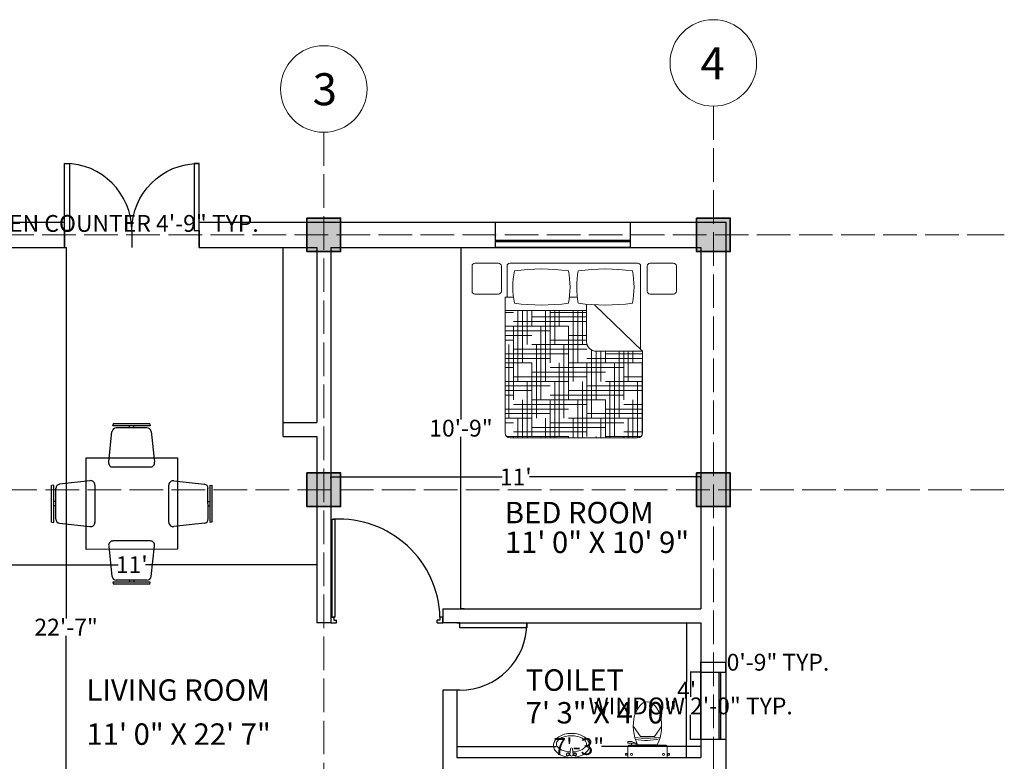
# Model space of a CAD drawing. Units: inches. Extents: x -113 to 5399, y -1393 to 3302.
# Tile 40 of 40: x 3412 to 3763, y 3038 to 3302. Entities that reach past the tile are written whole.
import ezdxf

# ---------------------------------------------------------------- set-up
doc = ezdxf.new("R2010")
doc.units = ezdxf.units.IN
doc.header["$MEASUREMENT"] = 0
doc.linetypes.add('ACAD_ISO02W100', pattern=[15, 12, -3])
for name, color, linetype, lineweight in [('A-ANNO-DIMS', 254, 'Continuous', 18), ('A-AREA-IDEN', 4, 'Continuous', 18), ('A-COLS', 7, 'Continuous', 35), ('A-FLOR-FIXT', 8, 'Continuous', 18), ('A-GRID-IDEN', 7, 'Continuous', 18), ('doors', 2, 'Continuous', 25), ('furniture', 131, 'Continuous', 18), ('GRIDS', 7, 'ACAD_ISO02W100', 13), ('walls', 1, 'Continuous', 25), ('windows', 3, 'Continuous', 25)]:
    doc.layers.add(name, color=color, linetype=linetype, lineweight=lineweight)
doc.layers.add('B-FURNITURE', color=22, linetype='Continuous')
doc.styles.get("Standard").update_dxf_attribs({"font": 'arial.ttf'})
doc.dimstyles.get("Standard").update_dxf_attribs({"dimtxt": 6, "dimasz": 0.18, "dimexe": 0.18, "dimexo": 0.0625, "dimgap": 0.09, "dimtad": 0, "dimtih": 1, "dimtoh": 1, "dimdec": 1, "dimzin": 0, "dimdsep": 46, "dimlunit": 4, "dimtxsty": 'Standard', "dimblk": 'ARCHTICK', "dimcen": 0.09, "dimadec": 0, "dimazin": 0, "dimtfac": 1, "dimtdec": 1, "dimtofl": 0, "dimtmove": 0, "dimatfit": 3, "dimfxl": 1, "dimtolj": 1, "dimtzin": 0, "dimarcsym": 0})

# ---------------------------------------------------------------- blocks, each defined once
blk = doc.blocks.new('*U2')
for p, q in [((0, 0), (0, -6)), ((24, 0), (24, -6))]:
    blk.add_line(p, q)
blk.add_lwpolyline([(0, 0), (0, 24), (1.75, 24), (1.75, 0)], close=True)
blk.add_arc((0, 0), 24, 0, 90)
blk = doc.blocks.new('*X4')
at = {"color": 0}
for p, q in [((4.359, 18.562), (4.359, 18.646)), ((4.453, 17.817), (4.453, 18.562)), ((4.5, 18), (4.5, 18.646)), ((4.5, 18.562), (5.25, 18.562)), ((4.547, 18.188), (4.547, 18.646)), ((4.594, 18.375), (4.594, 18.646)), ((4.641, 18.562), (4.641, 18.646)), ((4.687, 18.609), (5.437, 18.609)), ((4.734, 17.812), (4.734, 18.562)), ((4.781, 18), (4.781, 18.646)), ((4.828, 18.188), (4.828, 18.646)), ((4.875, 18.375), (4.875, 18.646)), ((4.922, 18.562), (4.922, 18.646)), ((5.016, 17.812), (5.016, 18.562)), ((5.062, 18), (5.062, 18.646)), ((5.109, 18.188), (5.109, 18.646)), ((5.156, 18.375), (5.156, 18.646)), ((5.203, 18.562), (5.203, 18.646)), ((5.297, 17.812), (5.297, 18.562)), ((5.344, 18), (5.344, 18.646)), ((5.391, 18.188), (5.391, 18.646)), ((5.437, 18.375), (5.437, 18.646)), ((5.484, 18.562), (5.484, 18.646)), ((5.578, 17.812), (5.578, 18.562)), ((5.625, 18), (5.625, 18.629)), ((5.625, 18.562), (5.637, 18.562)), ((4.34, 18.516), (5.062, 18.516)), ((4.34, 18.469), (4.875, 18.469)), ((5.25, 18.469), (5.637, 18.469)), ((5.437, 18.516), (5.637, 18.516)), ((4.34, 18.422), (4.687, 18.422)), ((4.34, 18.375), (4.5, 18.375)), ((4.406, 17.817), (4.406, 18.375)), ((4.687, 17.811), (4.687, 18.375)), ((4.875, 18.375), (5.625, 18.375)), ((4.969, 17.625), (4.969, 18.375)), ((5.062, 18.422), (5.637, 18.422)), ((5.25, 17.625), (5.25, 18.375)), ((5.531, 17.625), (5.531, 18.375)), ((4.5, 18.281), (5.25, 18.281)), ((4.687, 18.328), (5.437, 18.328)), ((5.625, 18.281), (5.637, 18.281)), ((4.34, 18.234), (5.062, 18.234)), ((4.34, 18.188), (4.875, 18.188)), ((4.359, 17.817), (4.359, 18.188)), ((4.641, 17.817), (4.641, 18.188)), ((4.922, 17.438), (4.922, 18.188)), ((5.203, 17.438), (5.203, 18.188)), ((5.25, 18.188), (5.637, 18.188)), ((5.437, 18.234), (5.637, 18.234)), ((5.484, 17.438), (5.484, 18.188)), ((4.34, 18.141), (4.687, 18.141)), ((4.34, 18.094), (4.5, 18.094)), ((4.875, 18.094), (5.625, 18.094)), ((5.062, 18.141), (5.637, 18.141)), ((4.5, 18), (5.25, 18)), ((4.594, 17.817), (4.594, 18)), ((4.687, 18.047), (5.437, 18.047)), ((4.875, 17.25), (4.875, 18)), ((5.156, 17.25), (5.156, 18)), ((5.437, 17.25), (5.437, 18)), ((5.625, 18), (5.637, 18)), ((4.34, 17.953), (5.062, 17.953)), ((4.34, 17.906), (4.875, 17.906)), ((4.34, 17.859), (4.687, 17.859)), ((5.062, 17.859), (5.637, 17.859)), ((5.25, 17.906), (5.637, 17.906)), ((5.437, 17.953), (5.637, 17.953)), ((4.742, 17.766), (5.437, 17.766)), ((4.828, 17.246), (4.828, 17.812)), ((4.875, 17.812), (5.625, 17.812)), ((5.109, 17.246), (5.109, 17.812)), ((5.391, 17.246), (5.391, 17.812)), ((4.755, 17.719), (5.25, 17.719)), ((4.755, 17.672), (5.062, 17.672)), ((5.437, 17.672), (5.637, 17.672)), ((5.625, 17.719), (5.637, 17.719)), ((4.755, 17.625), (4.875, 17.625)), ((4.781, 17.246), (4.781, 17.625)), ((5.062, 17.246), (5.062, 17.625)), ((5.062, 17.578), (5.637, 17.578)), ((5.25, 17.625), (5.637, 17.625)), ((5.344, 17.246), (5.344, 17.625)), ((5.625, 17.263), (5.625, 17.625)), ((4.755, 17.484), (5.437, 17.484)), ((4.875, 17.531), (5.625, 17.531)), ((4.755, 17.438), (5.25, 17.438)), ((4.755, 17.391), (5.062, 17.391)), ((5.016, 17.246), (5.016, 17.438)), ((5.297, 17.246), (5.297, 17.438)), ((5.437, 17.391), (5.637, 17.391)), ((5.578, 17.246), (5.578, 17.438)), ((5.625, 17.438), (5.637, 17.438)), ((4.755, 17.344), (4.875, 17.344)), ((5.062, 17.297), (5.637, 17.297)), ((5.25, 17.344), (5.637, 17.344)), ((4.875, 17.25), (5.608, 17.25)), ((4.969, 17.246), (4.969, 17.25)), ((5.25, 17.246), (5.25, 17.25)), ((5.531, 17.246), (5.531, 17.25))]:
    blk.add_line(p, q, dxfattribs=at)
blk = doc.blocks.new('MAT-P01')
for p, q in [((-0.021, 0.816), (-0.021, 0.56)), ((0.009, 0.846), (0.247, 0.846)), ((0.277, 0.816), (0.277, 0.56)), ((0.344, 0.816), (0.344, -0.032)), ((0.374, 0.846), (1.674, 0.846)), ((1.704, 0.816), (1.704, 0.5)), ((1.762, 0.816), (1.762, 0.56)), ((1.792, 0.846), (2.031, 0.846)), ((2.061, 0.816), (2.061, 0.56)), ((0.009, 0.53), (0.247, 0.53)), ((1.792, 0.53), (2.031, 0.53)), ((0.815, 0.423), (0.324, -0.051)), ((0.895, 0.429), (0.895, 0.049)), ((0.988, 0.5), (1.069, 0.5)), ((1.639, 0.5), (1.724, 0.5)), ((1.724, 0.5), (1.724, -0.884)), ((0.895, 0.364), (1.724, 0.364)), ((0.895, 0.364), (0.895, 0.049)), ((0.895, 0.364), (1.724, 0.364)), ((1.724, 0.364), (1.724, -0.884)), ((0.324, -0.051), (0.795, -0.051)), ((0.324, -0.051), (0.324, -0.884)), ((0.374, -0.934), (1.674, -0.934))]:
    blk.add_line(p, q)
for centre, radius, start, end in [((0.009, 0.816), 0.03, 90, 180), ((0.247, 0.816), 0.03, 0, 90), ((0.374, 0.816), 0.03, 90, 180), ((1.674, 0.816), 0.03, 0, 90), ((1.792, 0.816), 0.03, 90, 180), ((2.031, 0.816), 0.03, 0, 90), ((1.225, 0.603), 0.814, 168.373, 191.627), ((0.703, -1.144), 1.931, 81.8162, 98.1838), ((0.181, 0.603), 0.814, 348.373, 11.627), ((1.877, 0.603), 0.814, 168.373, 191.627), ((1.354, -1.144), 1.931, 81.8162, 98.1838), ((0.832, 0.603), 0.814, 348.373, 11.627), ((0.009, 0.56), 0.03, 180, 270), ((0.247, 0.56), 0.03, 270, 0), ((1.792, 0.56), 0.03, 180, 270), ((2.031, 0.56), 0.03, 270, 0), ((0.703, 2.35), 1.931, 261.8162, 278.1838), ((1.354, 2.35), 1.931, 261.8162, 278.1838), ((0.795, 0.049), 0.1, 270, 0), ((0.374, -0.884), 0.05, 180, 270), ((1.674, -0.884), 0.05, 270, 0)]:
    blk.add_arc(centre, radius, start, end)
at = {"rotation": 270}
blk.add_blockref('*X4', (-16.922, 4.704), dxfattribs=at)
blk = doc.blocks.new('A$C6ACA79D1')
at = {"layer": 'B-FURNITURE'}
for p, q in [((-0.503, 0.053), (-0.801, -0.244)), ((-0.483, 0.039), (-0.787, -0.264)), ((-0.503, 0.053), (-0.483, 0.039)), ((-0.429, 0), (-0.155, -0.22)), ((0.787, -0.259), (0.483, 0.044)), ((0.484, 0.043), (0.504, 0.058)), ((0.743, -0.249), (0.493, 0)), ((0.801, -0.239), (0.503, 0.059)), ((-0.493, -0.005), (-0.743, -0.254)), ((-0.601, -0.112), (-0.618, -0.095)), ((0.601, -0.107), (0.618, -0.09)), ((-0.635, -0.147), (-0.652, -0.13)), ((0.635, -0.142), (0.652, -0.124)), ((-0.786, -0.264), (-0.8, -0.244)), ((-0.148, -0.296), (-0.451, -0.599)), ((0.451, -0.594), (0.148, -0.291)), ((0.748, -0.313), (0.527, -0.588)), ((0.801, -0.239), (0.787, -0.259)), ((-0.148, -1.194), (-0.451, -0.891)), ((0.451, -0.896), (0.148, -1.199)), ((0.748, -1.177), (0.527, -0.902)), ((-0.786, -1.227), (-0.8, -1.247)), ((-0.483, -1.529), (-0.787, -1.226)), ((-0.493, -1.485), (-0.743, -1.236)), ((0.787, -1.231), (0.483, -1.535)), ((0.743, -1.241), (0.493, -1.49)), ((0.801, -1.251), (0.787, -1.231)), ((-0.503, -1.544), (-0.801, -1.246)), ((-0.635, -1.343), (-0.652, -1.361)), ((-0.429, -1.49), (-0.155, -1.27)), ((0.801, -1.251), (0.503, -1.549)), ((0.635, -1.349), (0.652, -1.366)), ((-0.601, -1.378), (-0.618, -1.395)), ((0.601, -1.383), (0.618, -1.4)), ((-0.503, -1.544), (-0.483, -1.529)), ((0.484, -1.534), (0.504, -1.548))]:
    blk.add_line(p, q, dxfattribs=at)
at = {"layer": 'B-FURNITURE', "ltscale": 300}
for p, q in [((0.155, -0.215), (0.429, 0.005)), ((-0.527, -0.593), (-0.748, -0.319)), ((-0.527, -0.897), (-0.748, -1.172)), ((0.155, -1.275), (0.429, -1.496))]:
    blk.add_line(p, q, dxfattribs=at)
blk.add_lwpolyline([(-0.742, -0.742), (0, 0), (0.742, -0.742), (0, -1.485)], close=True, dxfattribs=at)
at = {"layer": 'B-FURNITURE', "ltscale": 400}
for centre, start, end in [((-0.458, -0.04), 54.4069, 135), ((0.459, -0.036), 45, 125.5931), ((-0.706, -0.289), 135, 215.5931), ((0.707, -0.284), 324.4069, 45), ((-0.706, -1.201), 144.4069, 225), ((0.707, -1.206), 315, 35.5931), ((-0.458, -1.45), 225, 305.5931), ((0.459, -1.454), 234.4069, 315)]:
    blk.add_arc(centre, 0.0499, start, end, dxfattribs=at)
at = {"layer": 'B-FURNITURE', "ltscale": 300}
for centre, start, end in [((-0.184, -0.261), 315, 54.4069), ((0.184, -0.256), 125.5931, 225), ((-0.487, -0.564), 215.5931, 315), ((0.487, -0.559), 225, 324.4069), ((-0.487, -0.926), 45, 144.4069), ((0.487, -0.931), 35.5931, 135), ((-0.184, -1.229), 305.5931, 45), ((0.184, -1.234), 135, 234.4069)]:
    blk.add_arc(centre, 0.05, start, end, dxfattribs=at)
blk = doc.blocks.new('toilet-3')
at = {"color": 0, "linetype": 'ByBlock'}
for p, q in [((-0.281, -0.05), (-0.281, -0.069)), ((-0.281, -0.05), (-0.261, -0.05)), ((-0.281, -0.069), (-0.261, -0.069)), ((-0.261, -0.047), (-0.261, -0.072)), ((-0.261, -0.047), (-0.251, -0.047)), ((-0.261, -0.072), (-0.251, -0.072)), ((-0.251, -0.047), (-0.251, -0.072)), ((-0.25, -0.03), (-0.25, -0.165)), ((0.24, -0.02), (-0.24, -0.02)), ((0.25, -0.03), (0.25, -0.165)), ((0.261, -0.047), (0.251, -0.047)), ((0.251, -0.047), (0.251, -0.072)), ((0.261, -0.072), (0.251, -0.072)), ((0.261, -0.047), (0.261, -0.072)), ((0.281, -0.05), (0.261, -0.05)), ((0.281, -0.069), (0.261, -0.069)), ((0.281, -0.05), (0.281, -0.069)), ((-0.144, -0.2), (-0.25, -0.2)), ((-0.25, -0.2), (-0.25, -0.222)), ((-0.198, -0.222), (-0.25, -0.222)), ((0.24, -0.175), (-0.24, -0.175)), ((-0.202, -0.2), (-0.202, -0.175)), ((-0.198, -0.222), (-0.16, -0.207)), ((-0.16, -0.207), (-0.16, -0.2)), ((-0.144, -0.2), (-0.144, -0.175)), ((0.125, -0.182), (-0.125, -0.182)), ((-0.089, -0.287), (-0.18, -0.415)), ((0.089, -0.287), (-0.089, -0.287)), ((0.089, -0.287), (0.18, -0.415))]:
    blk.add_line(p, q, dxfattribs=at)
for centre in [(-0.205, -0.059), (0.205, -0.059)]:
    blk.add_circle(centre, 0.0125, dxfattribs=at)
for centre, radius, start, end in [((-0.24, -0.03), 0.01, 90, 180), ((0.24, -0.03), 0.01, 0, 90), ((-0.24, -0.165), 0.01, 180, 270), ((0.376, -0.424), 0.557, 154.2321, 193.6755), ((-0.005, -0.896), 0.659, 75.9276, 103.0204), ((-0.376, -0.424), 0.557, 346.3245, 25.7679), ((0.24, -0.165), 0.01, 270, 0), ((-0.013, -1.787), 1.521, 83.4552, 95.5271), ((0.262, -0.406), 0.452, 199.2942, 217.2549), ((-0.265, -0.4), 0.457, 322.2382, 340.1051), ((-0.001, -0.609), 0.12, 216.3794, 323.6206)]:
    blk.add_arc(centre, radius, start, end, dxfattribs=at)
blk = doc.blocks.new('wash-6')
at = {"color": 0, "linetype": 'ByBlock'}
for p, q in [((-0.036, -0.063), (-0.021, -0.18)), ((0.036, -0.063), (0.021, -0.18))]:
    blk.add_line(p, q, dxfattribs=at)
for centre, radius in [((-0.075, -0.062), 0.0325), ((-0.075, -0.062), 0.0263), ((0.075, -0.062), 0.0325), ((0.075, -0.062), 0.0263)]:
    blk.add_circle(centre, radius, dxfattribs=at)
for centre, radius, start, end in [((0, -0.56), 0.56, 90, 105.4371), ((-0.204, -0.25), 0.17, 148.1465, 180), ((-0.107, -0.311), 0.285, 123.6901, 148.1465), ((-0.114, -0.361), 0.225, 118.369, 142.5096), ((-0.042, -0.407), 0.401, 105.4371, 123.6901), ((-0.045, -0.488), 0.37, 102.6081, 118.369), ((0, -0.69), 0.576, 92.9466, 102.6081), ((0, -0.063), 0.0361, 0, 180), ((0, -0.18), 0.0215, 180, 0), ((0, -0.56), 0.56, 74.5629, 90), ((0, -0.69), 0.576, 77.3919, 87.0534), ((0.045, -0.488), 0.37, 61.631, 77.3919), ((0.042, -0.407), 0.401, 56.3099, 74.5629), ((0.114, -0.361), 0.225, 37.4904, 61.631), ((0.107, -0.311), 0.285, 31.8535, 56.3099), ((0.204, -0.25), 0.17, 0, 31.8535), ((-0.204, -0.25), 0.17, 180, 211.8535), ((-0.107, -0.189), 0.285, 211.8535, 236.3099), ((-0.217, -0.282), 0.0954, 142.5096, 180), ((-0.217, -0.282), 0.0954, 180, 217.4904), ((-0.114, -0.203), 0.225, 217.4904, 241.631), ((-0.045, -0.076), 0.37, 241.631, 257.3919), ((0.045, -0.076), 0.37, 282.6081, 298.369), ((0.114, -0.203), 0.225, 298.369, 322.5096), ((0.107, -0.189), 0.285, 303.6901, 328.1465), ((0.217, -0.282), 0.0954, 0, 37.4904), ((0.217, -0.282), 0.0954, 322.5096, 0), ((0.204, -0.25), 0.17, 328.1465, 0), ((-0.042, -0.092), 0.401, 236.3099, 254.5629), ((0, 0.06), 0.56, 254.5629, 270), ((0, 0.125), 0.576, 257.3919, 270), ((0, 0.125), 0.576, 270, 282.6081), ((0, 0.06), 0.56, 270, 285.4371), ((0.042, -0.092), 0.401, 285.4371, 303.6901)]:
    blk.add_arc(centre, radius, start, end, dxfattribs=at)
blk = doc.blocks.new('_ArchTick')
at = {"color": 0, "linetype": 'ByBlock', "const_width": 0.15}
blk.add_lwpolyline([(-0.5, -0.5), (0.5, 0.5)], dxfattribs=at)
blk = doc.blocks.new('*D125')
at = {"layer": 'A-ANNO-DIMS', "color": 0, "lineweight": -2, "transparency": 16777216}
for p, q in [((3427.61, 3221.06), (3428.31, 3221.06)), ((3428.13, 3221.06), (3428.13, 3088.66)), ((3428.13, 2950.06), (3428.13, 3082.46)), ((3430.16, 2950.06), (3427.95, 2950.06))]:
    blk.add_line(p, q, dxfattribs=at)
at = {"layer": 'Defpoints', "color": 0, "transparency": 16777216}
for p in [(3427.55, 3221.06), (3428.13, 3221.06), (3430.22, 2950.06)]:
    blk.add_point(p, dxfattribs=at)
at = {"layer": 'A-ANNO-DIMS', "color": 0, "lineweight": -2, "transparency": 16777216, "xscale": 0.18, "yscale": 0.18, "zscale": 0.18}
for p, rotation in [((3428.13, 3221.06), 90), ((3428.13, 2950.06), 270)]:
    blk.add_blockref('_ArchTick', p, dxfattribs=dict(at, rotation=rotation))
at = {"layer": 'A-ANNO-DIMS', "color": 0, "transparency": 16777216, "insert": (3428.13, 3085.56), "char_height": 6, "attachment_point": 5}
blk.add_mtext('\\A1;22\'-7"', dxfattribs=at)
blk = doc.blocks.new('*D126')
at = {"layer": 'A-ANNO-DIMS', "color": 0, "lineweight": -2, "transparency": 16777216}
for p, q in [((3385.55, 3108), (3385.55, 3107.65)), ((3385.55, 3107.83), (3446.65, 3107.83)), ((3517.55, 3107.83), (3456.45, 3107.83)), ((3517.55, 3108), (3517.55, 3107.65))]:
    blk.add_line(p, q, dxfattribs=at)
at = {"layer": 'Defpoints', "color": 0, "transparency": 16777216}
for p in [(3385.55, 3108.06), (3517.55, 3108.06), (3517.55, 3107.83)]:
    blk.add_point(p, dxfattribs=at)
at = {"layer": 'A-ANNO-DIMS', "color": 0, "lineweight": -2, "transparency": 16777216, "xscale": 0.18, "yscale": 0.18, "zscale": 0.18, "rotation": 180}
blk.add_blockref('_ArchTick', (3385.55, 3107.83), dxfattribs=at)
at = {"layer": 'A-ANNO-DIMS', "color": 0, "lineweight": -2, "transparency": 16777216, "xscale": 0.18, "yscale": 0.18, "zscale": 0.18}
blk.add_blockref('_ArchTick', (3517.55, 3107.83), dxfattribs=at)
at = {"layer": 'A-ANNO-DIMS', "color": 0, "transparency": 16777216, "insert": (3451.55, 3107.83), "char_height": 6, "attachment_point": 5}
blk.add_mtext("\\A1;11'", dxfattribs=at)
blk = doc.blocks.new('*D142')
at = {"layer": 'A-ANNO-DIMS', "color": 0, "lineweight": -2, "transparency": 16777216}
for p, q in [((3560.22, 3221.06), (3569.18, 3221.06)), ((3569, 3221.06), (3569, 3159.71)), ((3569, 3092.06), (3569, 3153.41)), ((3570.1, 3092.06), (3568.82, 3092.06))]:
    blk.add_line(p, q, dxfattribs=at)
at = {"layer": 'Defpoints', "color": 0, "transparency": 16777216}
for p in [(3560.16, 3221.06), (3569, 3092.06), (3570.17, 3092.06)]:
    blk.add_point(p, dxfattribs=at)
at = {"layer": 'A-ANNO-DIMS', "color": 0, "lineweight": -2, "transparency": 16777216, "xscale": 0.18, "yscale": 0.18, "zscale": 0.18}
for p, rotation in [((3569, 3221.06), 90), ((3569, 3092.06), 270)]:
    blk.add_blockref('_ArchTick', p, dxfattribs=dict(at, rotation=rotation))
at = {"layer": 'A-ANNO-DIMS', "color": 0, "transparency": 16777216, "insert": (3569, 3156.56), "char_height": 6, "attachment_point": 5}
blk.add_mtext('\\A1;10\'-9"', dxfattribs=at)
blk = doc.blocks.new('*D143')
at = {"layer": 'A-ANNO-DIMS', "color": 0, "lineweight": -2, "transparency": 16777216}
for p, q in [((3522.55, 3138.53), (3522.55, 3139.34)), ((3522.55, 3139.16), (3583.65, 3139.16)), ((3654.55, 3139.16), (3593.45, 3139.16)), ((3654.55, 3138.53), (3654.55, 3139.34))]:
    blk.add_line(p, q, dxfattribs=at)
at = {"layer": 'Defpoints', "color": 0, "transparency": 16777216}
for p in [(3522.55, 3139.16), (3522.55, 3138.46), (3654.55, 3138.46)]:
    blk.add_point(p, dxfattribs=at)
at = {"layer": 'A-ANNO-DIMS', "color": 0, "lineweight": -2, "transparency": 16777216, "xscale": 0.18, "yscale": 0.18, "zscale": 0.18, "rotation": 180}
blk.add_blockref('_ArchTick', (3522.55, 3139.16), dxfattribs=at)
at = {"layer": 'A-ANNO-DIMS', "color": 0, "lineweight": -2, "transparency": 16777216, "xscale": 0.18, "yscale": 0.18, "zscale": 0.18}
blk.add_blockref('_ArchTick', (3654.55, 3139.16), dxfattribs=at)
at = {"layer": 'A-ANNO-DIMS', "color": 0, "transparency": 16777216, "insert": (3588.55, 3139.16), "char_height": 6, "attachment_point": 5}
blk.add_mtext("\\A1;11'", dxfattribs=at)
blk = doc.blocks.new('*D150')
at = {"layer": 'A-ANNO-DIMS', "color": 0, "lineweight": -2, "transparency": 16777216}
for p, q in [((3649.29, 3087.06), (3649.7, 3087.06)), ((3649.52, 3087.06), (3649.52, 3066.15)), ((3649.52, 3039.06), (3649.52, 3059.97)), ((3649.29, 3039.06), (3649.7, 3039.06))]:
    blk.add_line(p, q, dxfattribs=at)
at = {"layer": 'Defpoints', "color": 0, "transparency": 16777216}
for p in [(3649.23, 3087.06), (3649.23, 3039.06), (3649.52, 3039.06)]:
    blk.add_point(p, dxfattribs=at)
at = {"layer": 'A-ANNO-DIMS', "color": 0, "lineweight": -2, "transparency": 16777216, "xscale": 0.18, "yscale": 0.18, "zscale": 0.18}
for p, rotation in [((3649.52, 3087.06), 90), ((3649.52, 3039.06), 270)]:
    blk.add_blockref('_ArchTick', p, dxfattribs=dict(at, rotation=rotation))
at = {"layer": 'A-ANNO-DIMS', "color": 0, "transparency": 16777216, "insert": (3649.52, 3063.06), "char_height": 6, "attachment_point": 5}
blk.add_mtext("\\A1;4'", dxfattribs=at)
blk = doc.blocks.new('*D151')
at = {"layer": 'A-ANNO-DIMS', "color": 0, "lineweight": -2, "transparency": 16777216}
for p, q in [((3567.55, 3043.39), (3567.55, 3042.77)), ((3567.55, 3042.95), (3603.01, 3042.95)), ((3654.55, 3042.95), (3619.09, 3042.95)), ((3654.55, 3043.39), (3654.55, 3042.77))]:
    blk.add_line(p, q, dxfattribs=at)
at = {"layer": 'Defpoints', "color": 0, "transparency": 16777216}
for p in [(3567.55, 3043.45), (3567.55, 3042.95), (3654.55, 3043.45)]:
    blk.add_point(p, dxfattribs=at)
at = {"layer": 'A-ANNO-DIMS', "color": 0, "lineweight": -2, "transparency": 16777216, "xscale": 0.18, "yscale": 0.18, "zscale": 0.18, "rotation": 180}
blk.add_blockref('_ArchTick', (3567.55, 3042.95), dxfattribs=at)
at = {"layer": 'A-ANNO-DIMS', "color": 0, "lineweight": -2, "transparency": 16777216, "xscale": 0.18, "yscale": 0.18, "zscale": 0.18}
blk.add_blockref('_ArchTick', (3654.55, 3042.95), dxfattribs=at)
at = {"layer": 'A-ANNO-DIMS', "color": 0, "transparency": 16777216, "insert": (3611.05, 3042.95), "char_height": 6, "attachment_point": 5}
blk.add_mtext('\\A1;7\'-3"', dxfattribs=at)
blk = doc.blocks.new('WIN-PLAN-48IN')
h = blk.add_hatch(color=256)
h.dxf.hatch_style = 1
h.paths.add_polyline_path([(48, 2.5), (0, 2.5), (0, 2), (48, 2)])
for p, q in [((0, 9), (48, 9)), ((0, 0), (0, 9)), ((48, 9), (48, 0)), ((48, 2.5), (0, 2.5)), ((48, 2), (0, 2)), ((48, 0), (0, 0))]:
    blk.add_line(p, q)
blk = doc.blocks.new('WIN-PLAN-24IN')
h = blk.add_hatch(color=256)
h.dxf.hatch_style = 1
h.paths.add_polyline_path([(6.5, 24), (6.5, 0), (7, 0), (7, 24)])
for p, q in [((0, 0), (0, 24)), ((0, 24), (9, 24)), ((6.5, 24), (6.5, 0)), ((7, 24), (7, 0)), ((9, 24), (9, 0)), ((9, 0), (0, 0))]:
    blk.add_line(p, q)
blk = doc.blocks.new('COLUMN-12IN-SQUARE')
h = blk.add_hatch(color=256)
h.dxf.hatch_style = 1
h.paths.add_polyline_path([(6, 6), (-6, 6), (-6, -6), (6, -6)])
blk.add_lwpolyline([(-6, 6), (6, 6), (6, -6), (-6, -6)], close=True)
blk = doc.blocks.new('DOOR-SINGLE-36IN-PLAN')
for p, q in [((0.5, 2), (0.5, 36.98)), ((0.5, 36.98), (1.5, 36.98)), ((1.5, 36.98), (1.5, 2)), ((0, 2), (0, 0)), ((0, 2), (1.04, 2)), ((1.5, 2), (0.5, 2)), ((1.04, 2), (1.04, 0.98)), ((1.04, 0.98), (2, 0.98)), ((2, 0), (2, 0.98)), ((38.96, 0.98), (38, 0.98)), ((38, 0), (38, 0.98)), ((40, 2), (38.96, 2)), ((38.96, 2), (38.96, 0.98)), ((40, 0), (40, 2)), ((0, 0), (2, 0)), ((0, 0), (2, 0)), ((38, 0), (40, 0))]:
    blk.add_line(p, q)
blk.add_arc((2.94, 0.99), 36.04, 1.6003, 93.0893)
blk = doc.blocks.new('GRID-BUBBLE-3')
blk.add_circle((0, 0), 15.44)
blk.add_text('3', height=11.45).set_placement((-3.95, -5.82))
blk = doc.blocks.new('GRID-BUBBLE-4')
blk.add_circle((0, 0), 15.44)
blk.add_text('4', height=11.45).set_placement((-4.57, -5.82))
blk = doc.blocks.new('*D181')
at = {"layer": 'A-ANNO-DIMS', "color": 0, "lineweight": -2, "transparency": 16777216}
for p, q in [((3323.4, 3221.12), (3323.4, 3229.81)), ((3323.4, 3229.63), (3380.55, 3229.63)), ((3380.55, 3221.12), (3380.55, 3229.81)), ((3380.55, 3229.63), (3380.73, 3229.63))]:
    blk.add_line(p, q, dxfattribs=at)
at = {"layer": 'Defpoints', "color": 0, "transparency": 16777216}
for p in [(3380.55, 3229.63), (3323.4, 3221.06), (3380.55, 3221.06)]:
    blk.add_point(p, dxfattribs=at)
at = {"layer": 'A-ANNO-DIMS', "color": 0, "lineweight": -2, "transparency": 16777216, "xscale": 0.18, "yscale": 0.18, "zscale": 0.18, "rotation": 180}
blk.add_blockref('_ArchTick', (3323.4, 3229.63), dxfattribs=at)
at = {"layer": 'A-ANNO-DIMS', "color": 0, "lineweight": -2, "transparency": 16777216, "xscale": 0.18, "yscale": 0.18, "zscale": 0.18}
blk.add_blockref('_ArchTick', (3380.55, 3229.63), dxfattribs=at)
at = {"layer": 'A-ANNO-DIMS', "color": 0, "transparency": 16777216, "insert": (3440.42, 3229.63), "char_height": 6, "attachment_point": 5}
blk.add_mtext('\\A1;KITCHEN COUNTER 4\'-9" TYP.', dxfattribs=at)
blk = doc.blocks.new('*D187')
at = {"layer": 'A-ANNO-DIMS', "color": 0, "lineweight": -2, "transparency": 16777216}
for p, q in [((3654.48, 3069.43), (3650.77, 3069.43)), ((3650.95, 3069.43), (3650.95, 3060.63)), ((3650.95, 3045.43), (3650.95, 3054.24)), ((3654.48, 3045.43), (3650.77, 3045.43))]:
    blk.add_line(p, q, dxfattribs=at)
at = {"layer": 'Defpoints', "color": 0, "transparency": 16777216}
for p in [(3650.95, 3069.43), (3654.55, 3069.43), (3654.55, 3045.43)]:
    blk.add_point(p, dxfattribs=at)
at = {"layer": 'A-ANNO-DIMS', "color": 0, "lineweight": -2, "transparency": 16777216, "xscale": 0.18, "yscale": 0.18, "zscale": 0.18}
for p, rotation in [((3650.95, 3069.43), 90), ((3650.95, 3045.43), 270)]:
    blk.add_blockref('_ArchTick', p, dxfattribs=dict(at, rotation=rotation))
at = {"layer": 'A-ANNO-DIMS', "color": 0, "transparency": 16777216, "insert": (3650.95, 3057.43), "char_height": 6, "attachment_point": 5}
blk.add_mtext('\\A1;WINDOW 2\'-0" TYP.', dxfattribs=at)
blk = doc.blocks.new('*D188')
at = {"layer": 'A-ANNO-DIMS', "color": 0, "lineweight": -2, "transparency": 16777216}
for p, q in [((3654.55, 3069.5), (3654.55, 3073.21)), ((3654.55, 3073.03), (3663.55, 3073.03)), ((3663.55, 3069.5), (3663.55, 3073.21)), ((3663.55, 3073.03), (3663.73, 3073.03))]:
    blk.add_line(p, q, dxfattribs=at)
at = {"layer": 'Defpoints', "color": 0, "transparency": 16777216}
for p in [(3663.55, 3073.03), (3654.55, 3069.43), (3663.55, 3069.43)]:
    blk.add_point(p, dxfattribs=at)
at = {"layer": 'A-ANNO-DIMS', "color": 0, "lineweight": -2, "transparency": 16777216, "xscale": 0.18, "yscale": 0.18, "zscale": 0.18, "rotation": 180}
blk.add_blockref('_ArchTick', (3654.55, 3073.03), dxfattribs=at)
at = {"layer": 'A-ANNO-DIMS', "color": 0, "lineweight": -2, "transparency": 16777216, "xscale": 0.18, "yscale": 0.18, "zscale": 0.18}
blk.add_blockref('_ArchTick', (3663.55, 3073.03), dxfattribs=at)
at = {"layer": 'A-ANNO-DIMS', "color": 0, "transparency": 16777216, "insert": (3682.1, 3073.03), "char_height": 6, "attachment_point": 5}
blk.add_mtext('\\A1;0\'-9" TYP.', dxfattribs=at)

msp = doc.modelspace()

# ---------------------------------------------------------------- linework, layer by layer
at = {"layer": 'GRIDS'}
for p, q in [((3659.05, 3271.46), (3659.05, 2498.02)), ((3520.05, 3262.17), (3520.05, 2490.34)), ((3104.61, 3225.56), (3753.5, 3225.56)), ((3753.5, 3225.56), (3762.86, 3225.56)), ((3105.74, 3134.56), (3762.86, 3134.56))]:
    msp.add_line(p, q, dxfattribs=at)
at = {"layer": 'walls'}
for p, q in [((3230.55, 3230.06), (3427.55, 3230.06)), ((3427.55, 3221.06), (3427.55, 3230.06)), ((3475.55, 3230.06), (3522.55, 3230.06)), ((3475.55, 3221.06), (3475.55, 3230.06)), ((3522.55, 3230.06), (3663.55, 3230.06)), ((3663.55, 3230.06), (3663.55, 2580.06)), ((3385.55, 3221.06), (3427.55, 3221.06)), ((3475.55, 3221.06), (3517.55, 3221.06)), ((3505.55, 3158.56), (3505.55, 3221.06)), ((3517.55, 3221.06), (3517.55, 3158.56)), ((3522.55, 3221.06), (3522.55, 3087.06)), ((3522.55, 3221.06), (3654.55, 3221.06)), ((3654.55, 3221.06), (3654.55, 3092.06)), ((3505.55, 3158.56), (3517.55, 3158.56)), ((3505.55, 3153.56), (3505.55, 3158.56)), ((3505.55, 3153.56), (3517.55, 3153.56)), ((3517.55, 3153.56), (3517.55, 3087.06)), ((3562.55, 3092.06), (3562.55, 3087.06)), ((3562.55, 3092.06), (3654.55, 3092.06)), ((3522.55, 3087.06), (3517.55, 3087.06)), ((3567.55, 3087.06), (3562.55, 3087.06)), ((3567.55, 3087.06), (3654.55, 3087.06)), ((3654.55, 3087.06), (3654.55, 3039.06)), ((3562.55, 3063.06), (3562.55, 3034.06)), ((3567.55, 3063.06), (3562.55, 3063.06)), ((3567.55, 3063.06), (3567.55, 3039.06)), ((3567.55, 3039.06), (3654.55, 3039.06))]:
    msp.add_line(p, q, dxfattribs=at)

# ---------------------------------------------------------------- block references
at = {"layer": 'A-COLS'}
for p in [(3520.05, 3225.56), (3659.05, 3225.56), (3520.05, 3134.56), (3659.05, 3134.56)]:
    msp.add_blockref('COLUMN-12IN-SQUARE', p, dxfattribs=at)
at = {"layer": 'A-FLOR-FIXT', "rotation": 180}
for name, p, xscale, yscale, zscale in [('toilet-3', (3635.55, 3038.5), -27.95492935005888, 27.95492935005888, 27.95492935005888), ('wash-6', (3608.42, 3039.06), -17.16666334294967, 17.16666334294967, 17.16666334294967)]:
    msp.add_blockref(name, p, dxfattribs=dict(at, xscale=xscale, yscale=yscale, zscale=zscale))
at = {"layer": 'A-GRID-IDEN'}
for name, p in [('GRID-BUBBLE-4', (3659.05, 3286.9)), ('GRID-BUBBLE-3', (3520.05, 3277.61))]:
    msp.add_blockref(name, p, dxfattribs=at)
at = {"layer": 'doors'}
for name, p in [('*U2', (3427.55, 3227.06)), ('DOOR-SINGLE-36IN-PLAN', (3522.55, 3087.06))]:
    msp.add_blockref(name, p, dxfattribs=at)
at = {"layer": 'doors', "xscale": -1}
msp.add_blockref('*U2', (3475.55, 3227.06), dxfattribs=at)
at = {"layer": 'doors', "rotation": 270}
msp.add_blockref('*U2', (3568.55, 3087.06), dxfattribs=at)
at = {"layer": 'furniture', "xscale": -35.02364872074636, "yscale": 35.02364872074636, "zscale": 35.02364872074636}
msp.add_blockref('MAT-P01', (3645.14, 3185.81), dxfattribs=at)
at = {"layer": 'furniture', "xscale": 31.0665876167328, "yscale": 31.0665876167328, "zscale": 31.0665876167328, "rotation": 314.9999999999397}
msp.add_blockref('A$C6ACA79D1', (3467.92, 3145.92), dxfattribs=at)
at = {"layer": 'windows'}
for name, p in [('WIN-PLAN-48IN', (3581.36, 3221.06)), ('WIN-PLAN-24IN', (3654.55, 3045.43))]:
    msp.add_blockref(name, p, dxfattribs=at)

# ---------------------------------------------------------------- texts
at = {"layer": 'A-AREA-IDEN'}
for s, height, p in [('BED ROOM', 7.647, (3584.66, 3122.6)), ('11\' 0" X 10\' 9"', 7.6473, (3584.66, 3112.01)), ('TOILET', 7.647, (3592.09, 3062.85)), ('LIVING ROOM', 7.6473, (3435.4, 3059.27)), ('7\' 3" X 4\' 0"', 7.6473, (3592.09, 3051.17)), ('11\' 0" X 22\' 7"', 7.6473, (3435.4, 3043.55))]:
    msp.add_text(s, height=height, dxfattribs=at).set_placement(p)

# ---------------------------------------------------------------- dimensions: what is measured, and where the dimension line sits
at = {"layer": 'A-ANNO-DIMS'}
for base, p1, p2, text, picture, middle in [((3380.5461, 3229.6314), (3323.398, 3221.0592), (3380.5461, 3221.0592), 'KITCHEN COUNTER <> TYP.', '*D181', (3440.415, 3229.6314)), ((3663.55, 3073.03), (3654.55, 3069.43), (3663.55, 3069.43), '<> TYP.', '*D188', (3682.1, 3073.03))]:
    dim = msp.add_linear_dim(base=base, p1=p1, p2=p2, text=text, dimstyle='Standard', override={"dimdec": 1, "dimlfac": 1, "dimrnd": 0, "dimzin": 1, "dimdsep": 46, "dimlunit": 4, "dimfrac": 2}, dxfattribs=at)
    dim.commit()
    dim.dimension.update_dxf_attribs({"geometry": picture, "text_midpoint": middle})
for base, p1, p2, picture, middle in [((3428.13, 3221.06), (3430.22, 2950.06), (3427.55, 3221.06), '*D125', (3428.13, 3085.56)), ((3569, 3092.06), (3560.16, 3221.06), (3570.17, 3092.06), '*D142', (3569, 3156.56)), ((3649.52, 3039.06), (3649.23, 3087.06), (3649.23, 3039.06), '*D150', (3649.52, 3063.06))]:
    dim = msp.add_linear_dim(base=base, p1=p1, p2=p2, angle=90, dimstyle='Standard', override={"dimclrd": 0, "dimclre": 0, "dimclrt": 0}, dxfattribs=at)
    dim.commit()
    dim.dimension.update_dxf_attribs({"geometry": picture, "text_midpoint": middle})
for base, p1, p2, picture, middle in [((3522.55, 3139.16), (3654.55, 3138.46), (3522.55, 3138.46), '*D143', (3588.55, 3139.16)), ((3517.55, 3107.83), (3385.55, 3108.06), (3517.55, 3108.06), '*D126', (3451.55, 3107.83)), ((3567.55, 3042.95), (3654.55, 3043.45), (3567.55, 3043.45), '*D151', (3611.05, 3042.95))]:
    dim = msp.add_linear_dim(base=base, p1=p1, p2=p2, dimstyle='Standard', override={"dimclrd": 0, "dimclre": 0, "dimclrt": 0}, dxfattribs=at)
    dim.commit()
    dim.dimension.update_dxf_attribs({"geometry": picture, "text_midpoint": middle})
dim = msp.add_linear_dim(base=(3650.95, 3069.43), p1=(3654.55, 3045.43), p2=(3654.55, 3069.43), angle=90, text='WINDOW <> TYP.', dimstyle='Standard', override={"dimdec": 1, "dimlfac": 1, "dimrnd": 0, "dimzin": 1, "dimdsep": 46, "dimlunit": 4, "dimfrac": 2}, dxfattribs=at)
dim.commit()
dim.dimension.update_dxf_attribs({"geometry": '*D187', "text_midpoint": (3650.95, 3057.43)})

doc.saveas('drawing.dxf')
